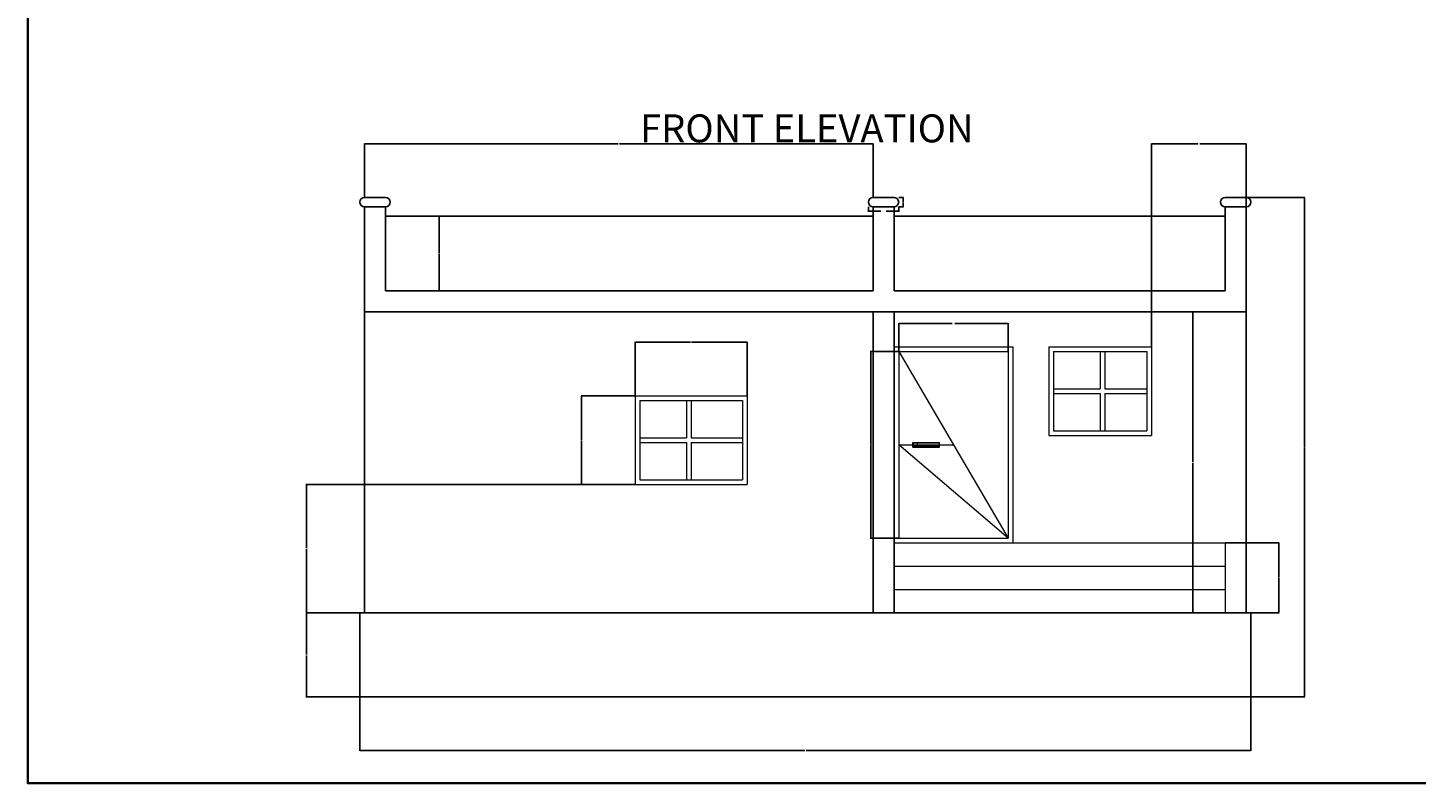
# Model space of a CAD drawing. Units: inches. Extents: x 2473 to 3664, y 1231 to 2079.
# Tile 1 of 8: x 2473 to 3069, y 1231 to 1555. Entities that reach past the tile are written whole.
import ezdxf

# ---------------------------------------------------------------- set-up
doc = ezdxf.new("R2010")
doc.units = ezdxf.units.IN
doc.linetypes.add('ACAD_ISO02W100', pattern=[15, 12, -3])
doc.layers.get('Defpoints').update_dxf_attribs({"linetype": 'ACAD_ISO02W100'})
for name, color, linetype, lineweight in [('A-ANNO-DIMS', 2, 'Continuous', 18), ('A-ANNO-TEXT', 4, 'Continuous', 25), ('A-ANNO-TTLB', 7, 'Continuous', 35), ('A-DOOR', 4, 'Continuous', 18), ('A-ELEV', 7, 'Continuous', 25), ('A-FLOR-STRS', 7, 'Continuous', 18), ('A-GLAZ', 3, 'Continuous', 18)]:
    doc.layers.add(name, color=color, linetype=linetype, lineweight=lineweight)
doc.styles.get("Standard").update_dxf_attribs({"font": 'arial.ttf'})
doc.dimstyles.get("Standard").update_dxf_attribs({"dimtxt": 0.18, "dimasz": 0.18, "dimexe": 0.18, "dimexo": 0.0625, "dimgap": 0.09, "dimtad": 0, "dimtih": 1, "dimtoh": 1, "dimdec": 4, "dimzin": 0, "dimdsep": 46, "dimtxsty": 'Standard', "dimcen": 0.09, "dimadec": 0, "dimazin": 0, "dimtfac": 1, "dimtdec": 4, "dimtofl": 0, "dimtmove": 0, "dimatfit": 3, "dimfxl": 1, "dimtolj": 1, "dimtzin": 0, "dimarcsym": 0})

# ---------------------------------------------------------------- blocks, each defined once
blk = doc.blocks.new('PARAPET-PIER-CAP')
for p, q in [((2, 4), (11, 4)), ((2, 0), (11, 0))]:
    blk.add_line(p, q)
for centre, start, end in [((2, 2), 90, 270), ((11, 2), 270, 90)]:
    blk.add_arc(centre, 2, start, end)
blk = doc.blocks.new('DOOR-LEAF-ELEV-47X80')
for p, q in [((0, 80), (47, 80)), ((0, 80), (0, 0)), ((0, 80), (47, 0)), ((47, 80), (47, 0)), ((0, 40), (23.5, 40)), ((47, 0), (0, 40)), ((6.03, 41), (17.47, 41)), ((6.03, 39), (6.03, 41)), ((6.03, 41), (6.33, 40.7)), ((6.03, 39), (6.33, 39.3)), ((6.03, 39), (17.47, 39)), ((17.17, 40.7), (6.33, 40.7)), ((6.33, 39.3), (6.33, 40.7)), ((17.17, 39.3), (6.33, 39.3)), ((8.03, 39.3), (8.03, 40.7)), ((17.47, 41), (17.17, 40.7)), ((17.47, 39), (17.17, 39.3)), ((17.47, 39), (17.47, 41)), ((0, 0), (47, 0))]:
    blk.add_line(p, q)
blk = doc.blocks.new('GLAZ-FOUR-LIGHT-ELEV')
for p, q in [((0, 38), (0, 0)), ((0, 38), (0.02, 38)), ((0.02, 38.03), (44.02, 38.03)), ((2, 36), (2, 2)), ((2, 36), (42.02, 36)), ((22, 36), (22, 20)), ((24, 36), (24, 20)), ((42.02, 36), (42.02, 2)), ((44.02, 38.03), (44.02, 0)), ((2, 20), (22, 20)), ((2, 18), (22, 18)), ((22, 18), (22, 2)), ((24, 20), (42.02, 20)), ((24, 18), (24, 2)), ((24, 18), (42.02, 18)), ((2, 2), (42.02, 2)), ((0, 0), (44.02, 0))]:
    blk.add_line(p, q)
blk = doc.blocks.new('*D23')
at = {"layer": 'A-ANNO-DIMS', "color": 0, "lineweight": -2, "transparency": 16777216}
for p, q in [((2833.66, 1478.21), (2833.66, 1476.14)), ((2833.84, 1476.32), (2839.01, 1476.32)), ((2846.48, 1476.32), (2841.31, 1476.32)), ((2846.66, 1478.21), (2846.66, 1476.14))]:
    blk.add_line(p, q, dxfattribs=at)
at = {"layer": 'A-ANNO-DIMS', "color": 0, "transparency": 16777216}
for points in [[(2833.84, 1476.35), (2833.84, 1476.29), (2833.66, 1476.32)], [(2846.48, 1476.35), (2846.48, 1476.29), (2846.66, 1476.32)]]:
    blk.add_solid(points, dxfattribs=at)
at = {"layer": 'Defpoints', "color": 0, "transparency": 16777216}
for p in [(2833.66, 1478.27), (2846.66, 1478.27), (2846.66, 1476.32)]:
    blk.add_point(p, dxfattribs=at)
at = {"layer": 'A-ANNO-DIMS', "color": 0, "transparency": 16777216, "insert": (2840.16, 1476.32), "char_height": 0.18, "attachment_point": 5}
blk.add_mtext('\\A1;PIER CAP 13 TYP.', dxfattribs=at)
blk = doc.blocks.new('*D24')
at = {"layer": 'A-ANNO-DIMS', "color": 0, "lineweight": -2, "transparency": 16777216}
for p, q in [((2846.72, 1482.27), (2848.79, 1482.27)), ((2846.72, 1478.27), (2848.79, 1478.27)), ((2848.61, 1482.09), (2848.61, 1480.45)), ((2848.61, 1478.45), (2848.61, 1480.09))]:
    blk.add_line(p, q, dxfattribs=at)
at = {"layer": 'A-ANNO-DIMS', "color": 0, "transparency": 16777216}
for points in [[(2848.58, 1482.09), (2848.64, 1482.09), (2848.61, 1482.27)], [(2848.58, 1478.45), (2848.64, 1478.45), (2848.61, 1478.27)]]:
    blk.add_solid(points, dxfattribs=at)
at = {"layer": 'Defpoints', "color": 0, "transparency": 16777216}
for p in [(2846.66, 1482.27), (2848.61, 1482.27), (2846.66, 1478.27)]:
    blk.add_point(p, dxfattribs=at)
at = {"layer": 'A-ANNO-DIMS', "color": 0, "transparency": 16777216, "insert": (2848.61, 1480.27), "char_height": 0.18, "attachment_point": 5}
blk.add_mtext('\\A1;4 TYP.', dxfattribs=at)
blk = doc.blocks.new('*D29')
at = {"layer": 'A-ANNO-DIMS', "color": 0, "lineweight": -2, "transparency": 16777216}
for p, q in [((2846.6, 1416.27), (2834.48, 1416.27)), ((2834.66, 1416.09), (2834.66, 1376.45)), ((2834.66, 1336.45), (2834.66, 1376.09)), ((2846.6, 1336.27), (2834.48, 1336.27))]:
    blk.add_line(p, q, dxfattribs=at)
at = {"layer": 'A-ANNO-DIMS', "color": 0, "transparency": 16777216}
for points in [[(2834.63, 1416.09), (2834.69, 1416.09), (2834.66, 1416.27)], [(2834.63, 1336.45), (2834.69, 1336.45), (2834.66, 1336.27)]]:
    blk.add_solid(points, dxfattribs=at)
at = {"layer": 'Defpoints', "color": 0, "transparency": 16777216}
for p in [(2834.66, 1416.27), (2846.66, 1416.27), (2846.66, 1336.27)]:
    blk.add_point(p, dxfattribs=at)
at = {"layer": 'A-ANNO-DIMS', "color": 0, "transparency": 16777216, "insert": (2834.66, 1376.27), "char_height": 0.18, "attachment_point": 5}
blk.add_mtext('\\A1;DOOR 80 TYP.', dxfattribs=at)
blk = doc.blocks.new('*D30')
at = {"layer": 'A-ANNO-DIMS', "color": 0, "lineweight": -2, "transparency": 16777216}
for p, q in [((2846.66, 1416.33), (2846.66, 1428.45)), ((2846.84, 1428.27), (2869.63, 1428.27)), ((2893.48, 1428.27), (2870.69, 1428.27)), ((2893.66, 1416.33), (2893.66, 1428.45))]:
    blk.add_line(p, q, dxfattribs=at)
at = {"layer": 'A-ANNO-DIMS', "color": 0, "transparency": 16777216}
for points in [[(2846.84, 1428.3), (2846.84, 1428.24), (2846.66, 1428.27)], [(2893.48, 1428.3), (2893.48, 1428.24), (2893.66, 1428.27)]]:
    blk.add_solid(points, dxfattribs=at)
at = {"layer": 'Defpoints', "color": 0, "transparency": 16777216}
for p in [(2893.66, 1428.27), (2846.66, 1416.27), (2893.66, 1416.27)]:
    blk.add_point(p, dxfattribs=at)
at = {"layer": 'A-ANNO-DIMS', "color": 0, "transparency": 16777216, "insert": (2870.16, 1428.27), "char_height": 0.18, "attachment_point": 5}
blk.add_mtext('\\A1;47 TYP.', dxfattribs=at)
blk = doc.blocks.new('*D79')
at = {"layer": 'A-ANNO-DIMS', "color": 0, "lineweight": -2, "transparency": 16777216}
for p, q in [((2615.66, 1268.21), (2615.66, 1245.14)), ((2997.66, 1268.21), (2997.66, 1245.14)), ((2615.84, 1245.32), (2806.37, 1245.32)), ((2997.48, 1245.32), (2806.95, 1245.32))]:
    blk.add_line(p, q, dxfattribs=at)
at = {"layer": 'A-ANNO-DIMS', "color": 0, "transparency": 16777216}
for points in [[(2615.84, 1245.35), (2615.84, 1245.29), (2615.66, 1245.32)], [(2997.48, 1245.35), (2997.48, 1245.29), (2997.66, 1245.32)]]:
    blk.add_solid(points, dxfattribs=at)
at = {"layer": 'Defpoints', "color": 0, "transparency": 16777216}
for p in [(2615.66, 1268.27), (2997.66, 1268.27), (2997.66, 1245.32)]:
    blk.add_point(p, dxfattribs=at)
at = {"layer": 'A-ANNO-DIMS', "color": 0, "transparency": 16777216, "insert": (2806.66, 1245.32), "char_height": 0.18, "attachment_point": 5}
blk.add_mtext('\\A1;382', dxfattribs=at)
blk = doc.blocks.new('*D80')
at = {"layer": 'A-ANNO-DIMS', "color": 0, "lineweight": -2, "transparency": 16777216}
for p, q in [((2995.72, 1482.27), (3020.79, 1482.27)), ((3020.61, 1482.09), (3020.61, 1375.45)), ((3020.61, 1268.45), (3020.61, 1375.09)), ((2997.72, 1268.27), (3020.79, 1268.27))]:
    blk.add_line(p, q, dxfattribs=at)
at = {"layer": 'A-ANNO-DIMS', "color": 0, "transparency": 16777216}
for points in [[(3020.58, 1482.09), (3020.64, 1482.09), (3020.61, 1482.27)], [(3020.58, 1268.45), (3020.64, 1268.45), (3020.61, 1268.27)]]:
    blk.add_solid(points, dxfattribs=at)
at = {"layer": 'Defpoints', "color": 0, "transparency": 16777216}
for p in [(2995.66, 1482.27), (3020.61, 1482.27), (2997.66, 1268.27)]:
    blk.add_point(p, dxfattribs=at)
at = {"layer": 'A-ANNO-DIMS', "color": 0, "transparency": 16777216, "insert": (3020.61, 1375.27), "char_height": 0.18, "attachment_point": 5}
blk.add_mtext('\\A1;214', dxfattribs=at)
blk = doc.blocks.new('*D81')
at = {"layer": 'A-ANNO-DIMS', "color": 0, "lineweight": -2, "transparency": 16777216}
for p, q in [((2615.6, 1304.27), (2592.53, 1304.27)), ((2592.71, 1304.09), (2592.71, 1286.45)), ((2592.71, 1268.45), (2592.71, 1286.09)), ((2615.6, 1268.27), (2592.53, 1268.27))]:
    blk.add_line(p, q, dxfattribs=at)
at = {"layer": 'A-ANNO-DIMS', "color": 0, "transparency": 16777216}
for points in [[(2592.68, 1304.09), (2592.74, 1304.09), (2592.71, 1304.27)], [(2592.68, 1268.45), (2592.74, 1268.45), (2592.71, 1268.27)]]:
    blk.add_solid(points, dxfattribs=at)
at = {"layer": 'Defpoints', "color": 0, "transparency": 16777216}
for p in [(2592.71, 1304.27), (2615.66, 1304.27), (2615.66, 1268.27)]:
    blk.add_point(p, dxfattribs=at)
at = {"layer": 'A-ANNO-DIMS', "color": 0, "transparency": 16777216, "insert": (2592.71, 1286.27), "char_height": 0.18, "attachment_point": 5}
blk.add_mtext('\\A1;36', dxfattribs=at)
blk = doc.blocks.new('*D82')
at = {"layer": 'A-ANNO-DIMS', "color": 0, "lineweight": -2, "transparency": 16777216}
for p, q in [((2733.6, 1359.27), (2592.53, 1359.27)), ((2592.71, 1359.09), (2592.71, 1331.95)), ((2592.71, 1304.45), (2592.71, 1331.59)), ((2615.6, 1304.27), (2592.53, 1304.27))]:
    blk.add_line(p, q, dxfattribs=at)
at = {"layer": 'A-ANNO-DIMS', "color": 0, "transparency": 16777216}
for points in [[(2592.68, 1359.09), (2592.74, 1359.09), (2592.71, 1359.27)], [(2592.68, 1304.45), (2592.74, 1304.45), (2592.71, 1304.27)]]:
    blk.add_solid(points, dxfattribs=at)
at = {"layer": 'Defpoints', "color": 0, "transparency": 16777216}
for p in [(2592.71, 1359.27), (2733.66, 1359.27), (2615.66, 1304.27)]:
    blk.add_point(p, dxfattribs=at)
at = {"layer": 'A-ANNO-DIMS', "color": 0, "transparency": 16777216, "insert": (2592.71, 1331.77), "char_height": 0.18, "attachment_point": 5}
blk.add_mtext('\\A1;55', dxfattribs=at)
blk = doc.blocks.new('*D83')
at = {"layer": 'A-ANNO-DIMS', "color": 0, "lineweight": -2, "transparency": 16777216}
for p, q in [((2986.72, 1334.27), (3009.79, 1334.27)), ((3009.61, 1334.09), (3009.61, 1319.45)), ((3009.61, 1304.45), (3009.61, 1319.09)), ((2986.72, 1304.27), (3009.79, 1304.27))]:
    blk.add_line(p, q, dxfattribs=at)
at = {"layer": 'A-ANNO-DIMS', "color": 0, "transparency": 16777216}
for points in [[(3009.58, 1334.09), (3009.64, 1334.09), (3009.61, 1334.27)], [(3009.58, 1304.45), (3009.64, 1304.45), (3009.61, 1304.27)]]:
    blk.add_solid(points, dxfattribs=at)
at = {"layer": 'Defpoints', "color": 0, "transparency": 16777216}
for p in [(2986.66, 1334.27), (2986.66, 1304.27), (3009.61, 1304.27)]:
    blk.add_point(p, dxfattribs=at)
at = {"layer": 'A-ANNO-DIMS', "color": 0, "transparency": 16777216, "insert": (3009.61, 1319.27), "char_height": 0.18, "attachment_point": 5}
blk.add_mtext('\\A1;30', dxfattribs=at)
blk = doc.blocks.new('*D84')
at = {"layer": 'A-ANNO-DIMS', "color": 0, "lineweight": -2, "transparency": 16777216}
for p, q in [((2995.6, 1433.27), (2972.53, 1433.27)), ((2972.71, 1433.09), (2972.71, 1368.95)), ((2972.71, 1304.45), (2972.71, 1368.59)), ((2995.6, 1304.27), (2972.53, 1304.27))]:
    blk.add_line(p, q, dxfattribs=at)
at = {"layer": 'A-ANNO-DIMS', "color": 0, "transparency": 16777216}
for points in [[(2972.68, 1433.09), (2972.74, 1433.09), (2972.71, 1433.27)], [(2972.68, 1304.45), (2972.74, 1304.45), (2972.71, 1304.27)]]:
    blk.add_solid(points, dxfattribs=at)
at = {"layer": 'Defpoints', "color": 0, "transparency": 16777216}
for p in [(2972.71, 1433.27), (2995.66, 1433.27), (2995.66, 1304.27)]:
    blk.add_point(p, dxfattribs=at)
at = {"layer": 'A-ANNO-DIMS', "color": 0, "transparency": 16777216, "insert": (2972.71, 1368.77), "char_height": 0.18, "attachment_point": 5}
blk.add_mtext('\\A1;129', dxfattribs=at)
blk = doc.blocks.new('*D85')
at = {"layer": 'A-ANNO-DIMS', "color": 0, "lineweight": -2, "transparency": 16777216}
for p, q in [((2617.66, 1482.33), (2617.66, 1505.4)), ((2617.84, 1505.22), (2726.37, 1505.22)), ((2835.48, 1505.22), (2726.95, 1505.22)), ((2835.66, 1482.33), (2835.66, 1505.4))]:
    blk.add_line(p, q, dxfattribs=at)
at = {"layer": 'A-ANNO-DIMS', "color": 0, "transparency": 16777216}
for points in [[(2617.84, 1505.25), (2617.84, 1505.19), (2617.66, 1505.22)], [(2835.48, 1505.25), (2835.48, 1505.19), (2835.66, 1505.22)]]:
    blk.add_solid(points, dxfattribs=at)
at = {"layer": 'Defpoints', "color": 0, "transparency": 16777216}
for p in [(2835.66, 1505.22), (2617.66, 1482.27), (2835.66, 1482.27)]:
    blk.add_point(p, dxfattribs=at)
at = {"layer": 'A-ANNO-DIMS', "color": 0, "transparency": 16777216, "insert": (2726.66, 1505.22), "char_height": 0.18, "attachment_point": 5}
blk.add_mtext('\\A1;218', dxfattribs=at)
blk = doc.blocks.new('*D86')
at = {"layer": 'A-ANNO-DIMS', "color": 0, "lineweight": -2, "transparency": 16777216}
for p, q in [((2626.72, 1474.27), (2649.79, 1474.27)), ((2649.61, 1474.09), (2649.61, 1458.45)), ((2649.61, 1442.45), (2649.61, 1458.09)), ((2626.72, 1442.27), (2649.79, 1442.27))]:
    blk.add_line(p, q, dxfattribs=at)
at = {"layer": 'A-ANNO-DIMS', "color": 0, "transparency": 16777216}
for points in [[(2649.58, 1474.09), (2649.64, 1474.09), (2649.61, 1474.27)], [(2649.58, 1442.45), (2649.64, 1442.45), (2649.61, 1442.27)]]:
    blk.add_solid(points, dxfattribs=at)
at = {"layer": 'Defpoints', "color": 0, "transparency": 16777216}
for p in [(2626.66, 1474.27), (2626.66, 1442.27), (2649.61, 1442.27)]:
    blk.add_point(p, dxfattribs=at)
at = {"layer": 'A-ANNO-DIMS', "color": 0, "transparency": 16777216, "insert": (2649.61, 1458.27), "char_height": 0.18, "attachment_point": 5}
blk.add_mtext('\\A1;32', dxfattribs=at)
blk = doc.blocks.new('*D87')
at = {"layer": 'A-ANNO-DIMS', "color": 0, "lineweight": -2, "transparency": 16777216}
for p, q in [((2733.66, 1397.33), (2733.66, 1420.4)), ((2733.84, 1420.22), (2757.44, 1420.22)), ((2781.48, 1420.22), (2757.88, 1420.22)), ((2781.66, 1397.33), (2781.66, 1420.4))]:
    blk.add_line(p, q, dxfattribs=at)
at = {"layer": 'A-ANNO-DIMS', "color": 0, "transparency": 16777216}
for points in [[(2733.84, 1420.25), (2733.84, 1420.19), (2733.66, 1420.22)], [(2781.48, 1420.25), (2781.48, 1420.19), (2781.66, 1420.22)]]:
    blk.add_solid(points, dxfattribs=at)
at = {"layer": 'Defpoints', "color": 0, "transparency": 16777216}
for p in [(2781.66, 1420.22), (2733.66, 1397.27), (2781.66, 1397.27)]:
    blk.add_point(p, dxfattribs=at)
at = {"layer": 'A-ANNO-DIMS', "color": 0, "transparency": 16777216, "insert": (2757.66, 1420.22), "char_height": 0.18, "attachment_point": 5}
blk.add_mtext('\\A1;48', dxfattribs=at)
blk = doc.blocks.new('*D88')
at = {"layer": 'A-ANNO-DIMS', "color": 0, "lineweight": -2, "transparency": 16777216}
for p, q in [((2733.6, 1397.27), (2710.53, 1397.27)), ((2710.71, 1397.09), (2710.71, 1378.45)), ((2710.71, 1359.45), (2710.71, 1378.09)), ((2733.6, 1359.27), (2710.53, 1359.27))]:
    blk.add_line(p, q, dxfattribs=at)
at = {"layer": 'A-ANNO-DIMS', "color": 0, "transparency": 16777216}
for points in [[(2710.68, 1397.09), (2710.74, 1397.09), (2710.71, 1397.27)], [(2710.68, 1359.45), (2710.74, 1359.45), (2710.71, 1359.27)]]:
    blk.add_solid(points, dxfattribs=at)
at = {"layer": 'Defpoints', "color": 0, "transparency": 16777216}
for p in [(2710.71, 1397.27), (2733.66, 1397.27), (2733.66, 1359.27)]:
    blk.add_point(p, dxfattribs=at)
at = {"layer": 'A-ANNO-DIMS', "color": 0, "transparency": 16777216, "insert": (2710.71, 1378.27), "char_height": 0.18, "attachment_point": 5}
blk.add_mtext('\\A1;38', dxfattribs=at)
blk = doc.blocks.new('*D89')
at = {"layer": 'A-ANNO-DIMS', "color": 0, "lineweight": -2, "transparency": 16777216}
for p, q in [((2955.01, 1418.33), (2955.01, 1505.4)), ((2955.19, 1505.22), (2974.94, 1505.22)), ((2995.48, 1505.22), (2975.73, 1505.22)), ((2995.66, 1433.33), (2995.66, 1505.4))]:
    blk.add_line(p, q, dxfattribs=at)
at = {"layer": 'A-ANNO-DIMS', "color": 0, "transparency": 16777216}
for points in [[(2955.19, 1505.25), (2955.19, 1505.19), (2955.01, 1505.22)], [(2995.48, 1505.25), (2995.48, 1505.19), (2995.66, 1505.22)]]:
    blk.add_solid(points, dxfattribs=at)
at = {"layer": 'Defpoints', "color": 0, "transparency": 16777216}
for p in [(2995.66, 1505.22), (2995.66, 1433.27), (2955.01, 1418.27)]:
    blk.add_point(p, dxfattribs=at)
at = {"layer": 'A-ANNO-DIMS', "color": 0, "transparency": 16777216, "insert": (2975.34, 1505.22), "char_height": 0.18, "attachment_point": 5}
blk.add_mtext('\\A1;40.65', dxfattribs=at)

msp = doc.modelspace()

# ---------------------------------------------------------------- linework, layer by layer
at = {"layer": 'A-ANNO-TTLB'}
msp.add_lwpolyline([(2473.2801, 2079.0861), (3663.7983, 2079.0861), (3663.7983, 1231.3065), (2473.2801, 1231.3065)], close=True, dxfattribs=at)
at = {"layer": 'A-DOOR'}
for p, q in [((2844.6604, 1418.2712), (2895.6604, 1418.2712)), ((2895.6604, 1418.2712), (2895.6604, 1334.2712))]:
    msp.add_line(p, q, dxfattribs=at)
at = {"layer": 'A-ELEV'}
for p, q in [((2617.6604, 1478.2712), (2617.6604, 1304.2712)), ((2626.6604, 1478.2712), (2626.6604, 1442.2712)), ((2835.6604, 1478.2712), (2835.6604, 1442.2712)), ((2844.6604, 1478.2712), (2844.6604, 1442.2712)), ((2986.6604, 1478.2712), (2986.6604, 1442.2712)), ((2995.6604, 1478.2712), (2995.6604, 1304.2712)), ((2626.6604, 1474.2712), (2835.6604, 1474.2712)), ((2844.6604, 1474.2712), (2986.6604, 1474.2712)), ((2626.6604, 1442.2712), (2835.6604, 1442.2712)), ((2844.6604, 1442.2712), (2986.6604, 1442.2712)), ((2617.6604, 1433.2712), (2995.6604, 1433.2712)), ((2626.6604, 1433.2712), (2835.6604, 1433.2712)), ((2835.6604, 1433.2712), (2835.6604, 1304.2712)), ((2844.6604, 1433.2712), (2844.6604, 1397.2712)), ((2844.6604, 1397.2712), (2844.6604, 1304.2712)), ((2615.6604, 1304.2712), (2997.6604, 1304.2712)), ((2615.6604, 1304.2712), (2615.6604, 1268.2712)), ((2997.6604, 1304.2712), (2997.6604, 1268.2712)), ((2615.6604, 1268.2712), (2997.6604, 1268.2712))]:
    msp.add_line(p, q, dxfattribs=at)
at = {"layer": 'A-FLOR-STRS'}
for p, q in [((2844.6604, 1334.2712), (2986.6604, 1334.2712)), ((2986.6604, 1334.2712), (2986.6604, 1304.2712)), ((2844.6604, 1324.2712), (2986.6604, 1324.2712)), ((2844.6604, 1314.2712), (2986.6604, 1314.2712))]:
    msp.add_line(p, q, dxfattribs=at)
at = {"layer": 'A-GLAZ'}
for p, q in [((2733.6604, 1397.2712), (2781.6604, 1397.2712)), ((2733.6604, 1397.2712), (2733.6604, 1359.2712)), ((2735.6604, 1395.2712), (2779.6604, 1395.2712)), ((2735.6604, 1395.2712), (2735.6604, 1361.2712)), ((2755.6604, 1395.2712), (2755.6604, 1379.2712)), ((2757.6604, 1395.2712), (2757.6604, 1379.2712)), ((2779.6604, 1395.2712), (2779.6604, 1361.2712)), ((2781.6604, 1397.2712), (2781.6604, 1359.2712)), ((2735.6604, 1379.2712), (2755.6604, 1379.2712)), ((2735.6604, 1377.2712), (2755.6604, 1377.2712)), ((2755.6604, 1377.2712), (2755.6604, 1361.2712)), ((2757.6604, 1379.2712), (2779.6604, 1379.2712)), ((2757.6604, 1377.2712), (2757.6604, 1361.2712)), ((2757.6604, 1377.2712), (2779.6604, 1377.2712)), ((2733.6604, 1359.2712), (2781.6604, 1359.2712)), ((2735.6604, 1361.2712), (2779.6604, 1361.2712))]:
    msp.add_line(p, q, dxfattribs=at)

# ---------------------------------------------------------------- block references
at = {"layer": 'A-DOOR'}
msp.add_blockref('DOOR-LEAF-ELEV-47X80', (2846.66, 1336.271), dxfattribs=at)
at = {"layer": 'A-ELEV'}
for p in [(2615.66, 1478.271), (2833.66, 1478.271), (2984.66, 1478.271)]:
    msp.add_blockref('PARAPET-PIER-CAP', p, dxfattribs=at)
at = {"layer": 'A-GLAZ'}
msp.add_blockref('GLAZ-FOUR-LIGHT-ELEV', (2910.994, 1380.239), dxfattribs=at)

# ---------------------------------------------------------------- texts
at = {"layer": 'A-ANNO-TEXT'}
msp.add_text('FRONT ELEVATION', height=12, dxfattribs=at).set_placement((2735.7755, 1505.8468))

# ---------------------------------------------------------------- dimensions: what is measured, and where the dimension line sits
at = {"layer": 'A-ANNO-DIMS'}
for base, p1, p2, override, picture, middle in [((2835.6604, 1505.2212), (2617.6604, 1482.2712), (2835.6604, 1482.2712), {"dimdec": 0, "dimlfac": 1, "dimrnd": 0, "dimzin": 0, "dimdsep": 46, "dimlunit": 2}, '*D85', (2726.6604, 1505.2212)), ((2995.6604, 1505.2212), (2955.0131, 1418.2712), (2995.6604, 1433.2712), {"dimdec": 2, "dimlfac": 1, "dimrnd": 0, "dimzin": 0, "dimdsep": 46, "dimlunit": 2}, '*D89', (2975.3368, 1505.2212)), ((2781.6604, 1420.2212), (2733.6604, 1397.2712), (2781.6604, 1397.2712), {"dimdec": 0, "dimlfac": 1, "dimrnd": 0, "dimzin": 0, "dimdsep": 46, "dimlunit": 2}, '*D87', (2757.6604, 1420.2212)), ((2997.6604, 1245.3212), (2615.6604, 1268.2712), (2997.6604, 1268.2712), {"dimdec": 0, "dimlfac": 1, "dimrnd": 0, "dimzin": 0, "dimdsep": 46, "dimlunit": 2}, '*D79', (2806.6604, 1245.3212))]:
    dim = msp.add_linear_dim(base=base, p1=p1, p2=p2, dimstyle='Standard', override=override, dxfattribs=at)
    dim.commit()
    dim.dimension.update_dxf_attribs({"geometry": picture, "text_midpoint": middle})
for base, p1, p2, text, picture, middle in [((2848.6104, 1482.2712), (2846.6604, 1478.2712), (2846.6604, 1482.2712), '<> TYP.', '*D24', (2848.6104, 1480.2712)), ((2834.6604, 1416.2712), (2846.6604, 1336.2712), (2846.6604, 1416.2712), 'DOOR <> TYP.', '*D29', (2834.6604, 1376.2712))]:
    dim = msp.add_linear_dim(base=base, p1=p1, p2=p2, angle=90, text=text, dimstyle='Standard', override={"dimdec": 0, "dimlfac": 1, "dimrnd": 0, "dimzin": 0, "dimdsep": 46, "dimlunit": 2}, dxfattribs=at)
    dim.commit()
    dim.dimension.update_dxf_attribs({"geometry": picture, "text_midpoint": middle})
for base, p1, p2, angle, picture, middle in [((3020.6104, 1482.2712), (2997.6604, 1268.2712), (2995.6604, 1482.2712), 90, '*D80', (3020.6104, 1375.2712)), ((2649.6104, 1442.2712), (2626.6604, 1474.2712), (2626.6604, 1442.2712), 270, '*D86', (2649.6104, 1458.2712)), ((2972.7104, 1433.2712), (2995.6604, 1304.2712), (2995.6604, 1433.2712), 90, '*D84', (2972.7104, 1368.7712)), ((2710.7104, 1397.2712), (2733.6604, 1359.2712), (2733.6604, 1397.2712), 90, '*D88', (2710.7104, 1378.2712)), ((2592.7104, 1359.2712), (2615.6604, 1304.2712), (2733.6604, 1359.2712), 90, '*D82', (2592.7104, 1331.7712)), ((3009.6104, 1304.2712), (2986.6604, 1334.2712), (2986.6604, 1304.2712), 270, '*D83', (3009.6104, 1319.2712)), ((2592.7104, 1304.2712), (2615.6604, 1268.2712), (2615.6604, 1304.2712), 90, '*D81', (2592.7104, 1286.2712))]:
    dim = msp.add_linear_dim(base=base, p1=p1, p2=p2, angle=angle, dimstyle='Standard', override={"dimdec": 0, "dimlfac": 1, "dimrnd": 0, "dimzin": 0, "dimdsep": 46, "dimlunit": 2}, dxfattribs=at)
    dim.commit()
    dim.dimension.update_dxf_attribs({"geometry": picture, "text_midpoint": middle})
for base, p1, p2, text, picture, middle in [((2846.6604, 1476.3212), (2833.6604, 1478.2712), (2846.6604, 1478.2712), 'PIER CAP <> TYP.', '*D23', (2840.1604, 1476.3212)), ((2893.6604, 1428.2712), (2846.6604, 1416.2712), (2893.6604, 1416.2712), '<> TYP.', '*D30', (2870.1604, 1428.2712))]:
    dim = msp.add_linear_dim(base=base, p1=p1, p2=p2, text=text, dimstyle='Standard', override={"dimdec": 0, "dimlfac": 1, "dimrnd": 0, "dimzin": 0, "dimdsep": 46, "dimlunit": 2}, dxfattribs=at)
    dim.commit()
    dim.dimension.update_dxf_attribs({"geometry": picture, "text_midpoint": middle})

doc.saveas('drawing.dxf')
